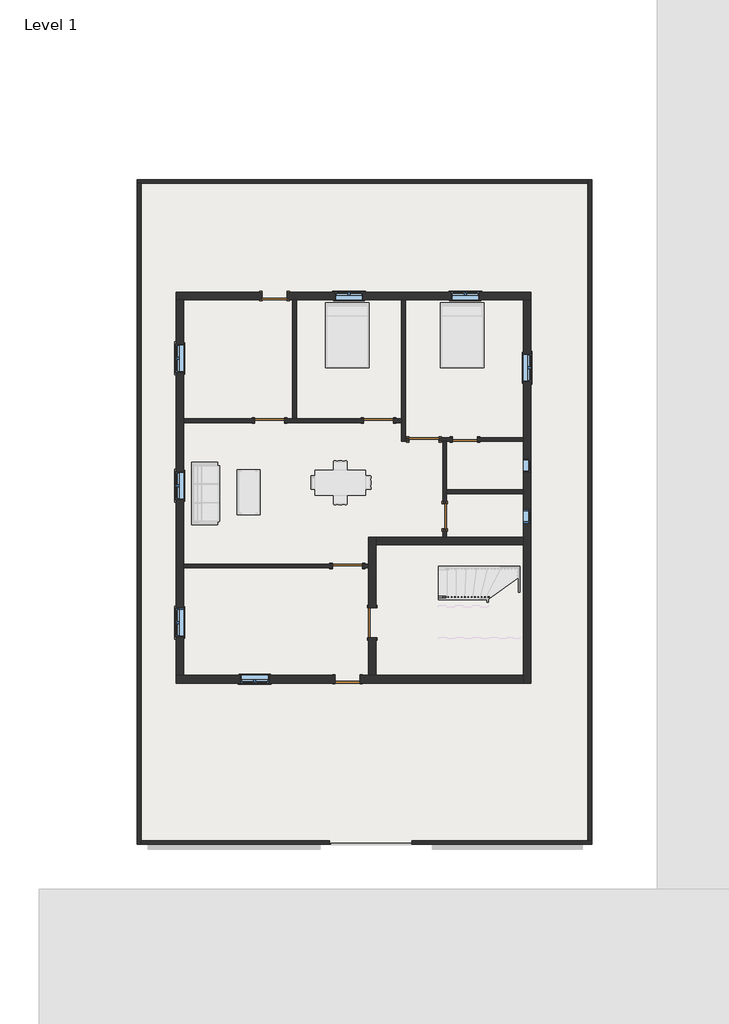
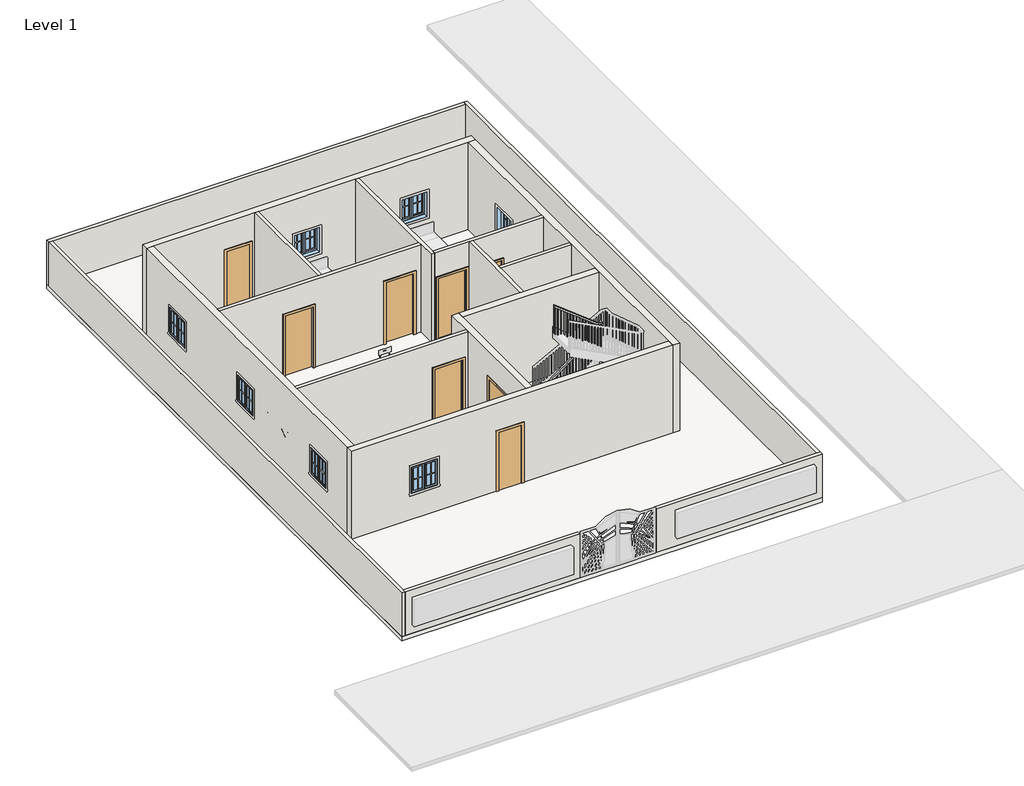
# One storey, part 1 of 2: 18 walls, 9 doors, 9 windows, 1 railing, 1 slab.
"""IFC4 building model written with IfcOpenShell, lengths in millimetres."""

from ifc_helpers import new_model, si_unit, frame, origin, origin_with_axes, place, context, project, spatial, polyline, outline, extrude, faceted_brep, transform, mapped, element, save
from components import door_85036156, door_d8f5dbb5, door_a1484949, door_e5f9f3c4, door_305aa2a5, door_0ca8825f, window_aa618e30, window_339605e1

model = new_model("IFC4")

# Units and contexts
model_context = context("Model", 3, world=origin())
ifc_project = project(units=[si_unit("LENGTHUNIT", "METRE", prefix="MILLI")], contexts=[model_context])

# Site, building, storey
site = spatial("IfcSite", under=ifc_project)
building = spatial("IfcBuilding", under=site)
storey = spatial("IfcBuildingStorey", under=building, Name="Level 1", Elevation=0.0)

# Doors
placement = place(None, origin())
door_shape = door_85036156(model_context)
element("IfcDoor", 1, ObjectType="Single-Flush : 30\" x 80\"", at=placement, inside=storey, context=model_context, shape_type="MappedRepresentation", body=[
    mapped(door_shape, transform((-3639.3817864, 7024.9034997, 0.0), x_axis=(1.0, 0.0, 0.0), y_axis=(0.0, 1.0, 0.0), z_axis=(0.0, 0.0, 1.0))),
])
door_2_shape = door_d8f5dbb5(model_context)
element("IfcDoor", 2, ObjectType="Single-Flush : 30\" x 80\"", at=placement, inside=storey, context=model_context, shape_type="MappedRepresentation", body=[
    mapped(door_2_shape, transform((2149.2782136, 2662.4534997, 0.0), x_axis=(-1.0, 0.0, 0.0), y_axis=(0.0, -1.0, 0.0), z_axis=(0.0, 0.0, 1.0))),
])
element("IfcDoor", 3, ObjectType="Single-Flush : 30\" x 80\"", at=placement, inside=storey, context=model_context, shape_type="MappedRepresentation", body=[
    mapped(door_2_shape, transform((1539.6782136, 322.4784997, 0.0), x_axis=(0.0, -1.0, 0.0), y_axis=(1.0, 0.0, 0.0), z_axis=(0.0, 0.0, 1.0))),
])
door_3_shape = door_a1484949(model_context)
element("IfcDoor", 4, ObjectType="Single-Flush : 30\" x 80\"", at=placement, inside=storey, context=model_context, shape_type="MappedRepresentation", body=[
    mapped(door_3_shape, transform((-1425.7717864, -4633.6965003, 0.0), x_axis=(-1.0, 0.0, 0.0), y_axis=(0.0, -1.0, 0.0), z_axis=(0.0, 0.0, 1.0))),
])
door_4_shape = door_e5f9f3c4(model_context)
element("IfcDoor", 5, ObjectType="Single-Flush : 36\" x 84\"", at=placement, inside=storey, context=model_context, shape_type="MappedRepresentation", body=[
    mapped(door_4_shape, transform((-477.0817864, 3233.9534997, 0.0), x_axis=(1.0, 0.0, 0.0), y_axis=(0.0, 1.0, 0.0), z_axis=(0.0, 0.0, 1.0))),
])
element("IfcDoor", 6, ObjectType="Single-Flush : 36\" x 84\"", at=placement, inside=storey, context=model_context, shape_type="MappedRepresentation", body=[
    mapped(door_4_shape, transform((-3791.7817864, 3233.9534997, 0.0), x_axis=(1.0, 0.0, 0.0), y_axis=(0.0, 1.0, 0.0), z_axis=(0.0, 0.0, 1.0))),
])
element("IfcDoor", 7, ObjectType="Single-Flush : 36\" x 84\"", at=placement, inside=storey, context=model_context, shape_type="MappedRepresentation", body=[
    mapped(door_4_shape, transform((-1425.7717864, -1188.1865003, 0.0), x_axis=(1.0, 0.0, 0.0), y_axis=(0.0, 1.0, 0.0), z_axis=(0.0, 0.0, 1.0))),
])
door_5_shape = door_305aa2a5(model_context)
element("IfcDoor", 8, ObjectType="Single-Flush : 36\" x 84\"", at=placement, inside=storey, context=model_context, shape_type="MappedRepresentation", body=[
    mapped(door_5_shape, transform((912.2982136, 2662.4534997, 0.0), x_axis=(-1.0, 0.0, 0.0), y_axis=(0.0, -1.0, 0.0), z_axis=(0.0, 0.0, 1.0))),
])
door_6_shape = door_0ca8825f(model_context)
element("IfcDoor", 9, ObjectType="Single-Flush : 36\" x 84\"", at=placement, inside=storey, context=model_context, shape_type="MappedRepresentation", body=[
    mapped(door_6_shape, transform((-663.7717864, -2910.9415003, 0.0), x_axis=(0.0, 1.0, 0.0), y_axis=(-1.0, 0.0, 0.0), z_axis=(0.0, 0.0, 1.0))),
])

# Railing
element("IfcRailing", 10, ObjectType="Handrail - Rectangular", at=placement, inside=storey, context=model_context, shape_type="SolidModel", body=[
    faceted_brep([(1342.8282136, -2108.9365003, 1083.7333333), (1342.8282136, -2108.9365003, 1019.4000346), (1342.8282136, -2159.7365003, 1019.4000346), (1342.8282136, -2159.7365003, 1083.7333333), (2794.3599055, -2108.9365003, 2211.6191036), (2845.1599055, -2108.9365003, 2186.7590024), (2845.1599055, -2159.7365003, 2186.7590024), (2794.3599055, -2159.7365003, 2211.6191036), (2794.3599055, -2108.9365003, 2414.6281882), (2845.1599055, -2108.9365003, 2363.8281882), (2845.1599055, -2159.7365003, 2363.8281882), (2794.3599055, -2159.7365003, 2414.6281882), (2921.3599055, -2108.9365003, 2414.6281882), (2921.3599055, -2108.9365003, 2363.8281882), (2870.5599055, -2159.7365003, 2363.8281882), (2870.5599055, -2159.7365003, 2414.6281882), (2921.3599055, -2235.9365003, 2414.6281882), (2921.3599055, -2265.0578342, 2363.8281882), (2870.5599055, -2265.0578342, 2363.8281882), (2870.5599055, -2235.9365003, 2414.6281882), (2921.3599055, -2362.9365003, 2631.5051451), (2921.3599055, -2413.7365003, 2617.7256424), (2870.5599055, -2413.7365003, 2617.7256424), (2870.5599055, -2362.9365003, 2631.5051451), (2921.3599055, -2362.9365003, 2834.5142297), (2921.3599055, -2413.7365003, 2783.7142297), (2870.5599055, -2413.7365003, 2783.7142297), (2870.5599055, -2362.9365003, 2834.5142297), (2921.3599055, -2489.9365003, 2834.5142297), (2921.3599055, -2489.9365003, 2783.7142297), (2870.5599055, -2439.1365003, 2783.7142297), (2870.5599055, -2439.1365003, 2834.5142297), (2794.3599055, -2489.9365003, 2834.5142297), (2776.9432376, -2489.9365003, 2783.7142297), (2776.9432376, -2439.1365003, 2783.7142297), (2794.3599055, -2439.1365003, 2834.5142297), (1342.8282136, -2489.9365003, 3962.4), (1342.8282136, -2439.1365003, 3962.4), (1342.8282136, -2439.1365003, 3898.0667013), (1342.8282136, -2489.9365003, 3898.0667013)], [[[0, 1, 2, 3]], [[1, 0, 4, 5]], [[2, 1, 5, 6]], [[3, 2, 6, 7]], [[0, 3, 7, 4]], [[5, 4, 8, 9]], [[6, 5, 9, 10]], [[7, 6, 10, 11]], [[4, 7, 11, 8]], [[9, 8, 12, 13]], [[10, 9, 13, 14]], [[11, 10, 14, 15]], [[8, 11, 15, 12]], [[13, 12, 16, 17]], [[14, 13, 17, 18]], [[15, 14, 18, 19]], [[12, 15, 19, 16]], [[17, 16, 20, 21]], [[18, 17, 21, 22]], [[19, 18, 22, 23]], [[16, 19, 23, 20]], [[21, 20, 24, 25]], [[22, 21, 25, 26]], [[23, 22, 26, 27]], [[20, 23, 27, 24]], [[25, 24, 28, 29]], [[26, 25, 29, 30]], [[27, 26, 30, 31]], [[24, 27, 31, 28]], [[29, 28, 32, 33]], [[30, 29, 33, 34]], [[31, 30, 34, 35]], [[28, 31, 35, 32]], [[36, 37, 38, 39]], [[33, 32, 36, 39]], [[34, 33, 39, 38]], [[35, 34, 38, 37]], [[32, 35, 37, 36]]]),
    extrude(outline(polyline([(3868.0292361, 1381.4849055), (3882.8316852, 1362.4349055), (2878.6666667, 1362.4349055), (2878.6666667, 1381.4849055), (3868.0292361, 1381.4849055)])), frame((0.0, -2474.0615003, 0.0), z_axis=(0.0, 1.0, 0.0), x_axis=(0.0, 0.0, 1.0)), (0.0, 0.0, 1.0), 19.05),
    extrude(outline(polyline([(3789.0828411, 1483.0849055), (3803.8852902, 1464.0349055), (2878.6666667, 1464.0349055), (2878.6666667, 1483.0849055), (3789.0828411, 1483.0849055)])), frame((0.0, -2474.0615003, 0.0), z_axis=(0.0, 1.0, 0.0), x_axis=(0.0, 0.0, 1.0)), (0.0, 0.0, 1.0), 19.05),
    extrude(outline(polyline([(3710.1364462, 1584.6849055), (3724.9388952, 1565.6349055), (2878.6666667, 1565.6349055), (2878.6666667, 1584.6849055), (3710.1364462, 1584.6849055)])), frame((0.0, -2474.0615003, 0.0), z_axis=(0.0, 1.0, 0.0), x_axis=(0.0, 0.0, 1.0)), (0.0, 0.0, 1.0), 19.05),
    extrude(outline(polyline([(3631.1900512, 1686.2849055), (3645.9925003, 1667.2349055), (2709.3333333, 1667.2349055), (2709.3333333, 1686.2849055), (3631.1900512, 1686.2849055)])), frame((0.0, -2474.0615003, 0.0), z_axis=(0.0, 1.0, 0.0), x_axis=(0.0, 0.0, 1.0)), (0.0, 0.0, 1.0), 19.05),
    extrude(outline(polyline([(3552.2436562, 1787.8849055), (3567.0461053, 1768.8349055), (2709.3333333, 1768.8349055), (2709.3333333, 1787.8849055), (3552.2436562, 1787.8849055)])), frame((0.0, -2474.0615003, 0.0), z_axis=(0.0, 1.0, 0.0), x_axis=(0.0, 0.0, 1.0)), (0.0, 0.0, 1.0), 19.05),
    extrude(outline(polyline([(3473.2972613, 1889.4849055), (3488.0997103, 1870.4349055), (2709.3333333, 1870.4349055), (2709.3333333, 1889.4849055), (3473.2972613, 1889.4849055)])), frame((0.0, -2474.0615003, 0.0), z_axis=(0.0, 1.0, 0.0), x_axis=(0.0, 0.0, 1.0)), (0.0, 0.0, 1.0), 19.05),
    extrude(outline(polyline([(3394.3508663, 1991.0849055), (3409.1533154, 1972.0349055), (2540.0, 1972.0349055), (2540.0, 1991.0849055), (3394.3508663, 1991.0849055)])), frame((0.0, -2474.0615003, 0.0), z_axis=(0.0, 1.0, 0.0), x_axis=(0.0, 0.0, 1.0)), (0.0, 0.0, 1.0), 19.05),
    extrude(outline(polyline([(3315.4044713, 2092.6849055), (3330.2069204, 2073.6349055), (2540.0, 2073.6349055), (2540.0, 2092.6849055), (3315.4044713, 2092.6849055)])), frame((0.0, -2474.0615003, 0.0), z_axis=(0.0, 1.0, 0.0), x_axis=(0.0, 0.0, 1.0)), (0.0, 0.0, 1.0), 19.05),
    extrude(outline(polyline([(3236.4580764, 2194.2849055), (3251.2605254, 2175.2349055), (2370.6666667, 2175.2349055), (2370.6666667, 2194.2849055), (3236.4580764, 2194.2849055)])), frame((0.0, -2474.0615003, 0.0), z_axis=(0.0, 1.0, 0.0), x_axis=(0.0, 0.0, 1.0)), (0.0, 0.0, 1.0), 19.05),
    extrude(outline(polyline([(3157.5116814, 2295.8849055), (3172.3141304, 2276.8349055), (2370.6666667, 2276.8349055), (2370.6666667, 2295.8849055), (3157.5116814, 2295.8849055)])), frame((0.0, -2474.0615003, 0.0), z_axis=(0.0, 1.0, 0.0), x_axis=(0.0, 0.0, 1.0)), (0.0, 0.0, 1.0), 19.05),
    extrude(outline(polyline([(3078.5652864, 2397.4849055), (3093.3677355, 2378.4349055), (2370.6666667, 2378.4349055), (2370.6666667, 2397.4849055), (3078.5652864, 2397.4849055)])), frame((0.0, -2474.0615003, 0.0), z_axis=(0.0, 1.0, 0.0), x_axis=(0.0, 0.0, 1.0)), (0.0, 0.0, 1.0), 19.05),
    extrude(outline(polyline([(2999.6188914, 2499.0849055), (3014.4213405, 2480.0349055), (2201.3333333, 2480.0349055), (2201.3333333, 2499.0849055), (2999.6188914, 2499.0849055)])), frame((0.0, -2474.0615003, 0.0), z_axis=(0.0, 1.0, 0.0), x_axis=(0.0, 0.0, 1.0)), (0.0, 0.0, 1.0), 19.05),
    extrude(outline(polyline([(2920.6724965, 2600.6849055), (2935.4749455, 2581.6349055), (2201.3333333, 2581.6349055), (2201.3333333, 2600.6849055), (2920.6724965, 2600.6849055)])), frame((0.0, -2474.0615003, 0.0), z_axis=(0.0, 1.0, 0.0), x_axis=(0.0, 0.0, 1.0)), (0.0, 0.0, 1.0), 19.05),
    extrude(outline(polyline([(2841.7261015, 2702.2849055), (2856.5285506, 2683.2349055), (2032.0, 2683.2349055), (2032.0, 2702.2849055), (2841.7261015, 2702.2849055)])), frame((0.0, -2474.0615003, 0.0), z_axis=(0.0, 1.0, 0.0), x_axis=(0.0, 0.0, 1.0)), (0.0, 0.0, 1.0), 19.05),
    extrude(outline(polyline([(2762.7797065, 2803.8849055), (2777.5821556, 2784.8349055), (2032.0, 2784.8349055), (2032.0, 2803.8849055), (2762.7797065, 2803.8849055)])), frame((0.0, -2474.0615003, 0.0), z_axis=(0.0, 1.0, 0.0), x_axis=(0.0, 0.0, 1.0)), (0.0, 0.0, 1.0), 19.05),
    extrude(outline(polyline([(2886.4349055, -2429.6115003), (2905.4849055, -2429.6115003), (2905.4849055, -2448.6615003), (2886.4349055, -2448.6615003), (2886.4349055, -2429.6115003)])), frame((0.0, 0.0, 1693.3333333), z_axis=(0.0, 0.0, 1.0), x_axis=(1.0, 0.0, 0.0)), (0.0, 0.0, 1.0), 1090.3808964),
    extrude(outline(polyline([(-2347.0615003, 2503.86524), (-2328.0115003, 2471.3336964), (-2328.0115003, 1524.0), (-2347.0615003, 1524.0), (-2347.0615003, 2503.86524)])), frame((2886.4349055, 0.0, 0.0), z_axis=(1.0, 0.0, 0.0), x_axis=(0.0, 1.0, 0.0)), (0.0, 0.0, 1.0), 19.05),
    extrude(outline(polyline([(-2245.4615003, 2330.3636744), (-2226.4115003, 2297.8321309), (-2226.4115003, 1354.6666667), (-2245.4615003, 1354.6666667), (-2245.4615003, 2330.3636744)])), frame((2886.4349055, 0.0, 0.0), z_axis=(1.0, 0.0, 0.0), x_axis=(0.0, 1.0, 0.0)), (0.0, 0.0, 1.0), 19.05),
    extrude(outline(polyline([(2857.3032136, -2143.8615003), (2857.3032136, -2124.8115003), (2876.3532136, -2124.8115003), (2876.3532136, -2143.8615003), (2857.3032136, -2143.8615003)])), frame((0.0, 0.0, 1185.3333333), z_axis=(0.0, 0.0, 1.0), x_axis=(1.0, 0.0, 0.0)), (0.0, 0.0, 1.0), 1178.4948549),
    extrude(outline(polyline([(2132.0507888, 2774.7532136), (2117.2483397, 2755.7032136), (1016.0, 2755.7032136), (1016.0, 2774.7532136), (2132.0507888, 2774.7532136)])), frame((0.0, -2143.8615003, 0.0), z_axis=(0.0, 1.0, 0.0), x_axis=(0.0, 0.0, 1.0)), (0.0, 0.0, 1.0), 19.05),
    extrude(outline(polyline([(2053.1043938, 2673.1532136), (2038.3019447, 2654.1032136), (1016.0, 2654.1032136), (1016.0, 2673.1532136), (2053.1043938, 2673.1532136)])), frame((0.0, -2143.8615003, 0.0), z_axis=(0.0, 1.0, 0.0), x_axis=(0.0, 0.0, 1.0)), (0.0, 0.0, 1.0), 19.05),
    extrude(outline(polyline([(1974.1579988, 2571.5532136), (1959.3555498, 2552.5032136), (846.6666667, 2552.5032136), (846.6666667, 2571.5532136), (1974.1579988, 2571.5532136)])), frame((0.0, -2143.8615003, 0.0), z_axis=(0.0, 1.0, 0.0), x_axis=(0.0, 0.0, 1.0)), (0.0, 0.0, 1.0), 19.05),
    extrude(outline(polyline([(1895.2116039, 2469.9532136), (1880.4091548, 2450.9032136), (846.6666667, 2450.9032136), (846.6666667, 2469.9532136), (1895.2116039, 2469.9532136)])), frame((0.0, -2143.8615003, 0.0), z_axis=(0.0, 1.0, 0.0), x_axis=(0.0, 0.0, 1.0)), (0.0, 0.0, 1.0), 19.05),
    extrude(outline(polyline([(1816.2652089, 2368.3532136), (1801.4627598, 2349.3032136), (677.3333333, 2349.3032136), (677.3333333, 2368.3532136), (1816.2652089, 2368.3532136)])), frame((0.0, -2143.8615003, 0.0), z_axis=(0.0, 1.0, 0.0), x_axis=(0.0, 0.0, 1.0)), (0.0, 0.0, 1.0), 19.05),
    extrude(outline(polyline([(1737.3188139, 2266.7532136), (1722.5163649, 2247.7032136), (677.3333333, 2247.7032136), (677.3333333, 2266.7532136), (1737.3188139, 2266.7532136)])), frame((0.0, -2143.8615003, 0.0), z_axis=(0.0, 1.0, 0.0), x_axis=(0.0, 0.0, 1.0)), (0.0, 0.0, 1.0), 19.05),
    extrude(outline(polyline([(1658.3724189, 2165.1532136), (1643.5699699, 2146.1032136), (508.0, 2146.1032136), (508.0, 2165.1532136), (1658.3724189, 2165.1532136)])), frame((0.0, -2143.8615003, 0.0), z_axis=(0.0, 1.0, 0.0), x_axis=(0.0, 0.0, 1.0)), (0.0, 0.0, 1.0), 19.05),
    extrude(outline(polyline([(1579.426024, 2063.5532136), (1564.6235749, 2044.5032136), (508.0, 2044.5032136), (508.0, 2063.5532136), (1579.426024, 2063.5532136)])), frame((0.0, -2143.8615003, 0.0), z_axis=(0.0, 1.0, 0.0), x_axis=(0.0, 0.0, 1.0)), (0.0, 0.0, 1.0), 19.05),
    extrude(outline(polyline([(1500.479629, 1961.9532136), (1485.6771799, 1942.9032136), (508.0, 1942.9032136), (508.0, 1961.9532136), (1500.479629, 1961.9532136)])), frame((0.0, -2143.8615003, 0.0), z_axis=(0.0, 1.0, 0.0), x_axis=(0.0, 0.0, 1.0)), (0.0, 0.0, 1.0), 19.05),
    extrude(outline(polyline([(1421.533234, 1860.3532136), (1406.730785, 1841.3032136), (338.6666667, 1841.3032136), (338.6666667, 1860.3532136), (1421.533234, 1860.3532136)])), frame((0.0, -2143.8615003, 0.0), z_axis=(0.0, 1.0, 0.0), x_axis=(0.0, 0.0, 1.0)), (0.0, 0.0, 1.0), 19.05),
    extrude(outline(polyline([(1342.5868391, 1758.7532136), (1327.78439, 1739.7032136), (338.6666667, 1739.7032136), (338.6666667, 1758.7532136), (1342.5868391, 1758.7532136)])), frame((0.0, -2143.8615003, 0.0), z_axis=(0.0, 1.0, 0.0), x_axis=(0.0, 0.0, 1.0)), (0.0, 0.0, 1.0), 19.05),
    extrude(outline(polyline([(1263.6404441, 1657.1532136), (1248.837995, 1638.1032136), (338.6666667, 1638.1032136), (338.6666667, 1657.1532136), (1263.6404441, 1657.1532136)])), frame((0.0, -2143.8615003, 0.0), z_axis=(0.0, 1.0, 0.0), x_axis=(0.0, 0.0, 1.0)), (0.0, 0.0, 1.0), 19.05),
    extrude(outline(polyline([(1184.6940491, 1555.5532136), (1169.8916001, 1536.5032136), (169.3333333, 1536.5032136), (169.3333333, 1555.5532136), (1184.6940491, 1555.5532136)])), frame((0.0, -2143.8615003, 0.0), z_axis=(0.0, 1.0, 0.0), x_axis=(0.0, 0.0, 1.0)), (0.0, 0.0, 1.0), 19.05),
    extrude(outline(polyline([(1105.7476541, 1453.9532136), (1090.9452051, 1434.9032136), (169.3333333, 1434.9032136), (169.3333333, 1453.9532136), (1105.7476541, 1453.9532136)])), frame((0.0, -2143.8615003, 0.0), z_axis=(0.0, 1.0, 0.0), x_axis=(0.0, 0.0, 1.0)), (0.0, 0.0, 1.0), 19.05),
    extrude(outline(polyline([(2886.4349055, -2455.0115003), (2905.4849055, -2455.0115003), (2905.4849055, -2474.0615003), (2886.4349055, -2474.0615003), (2886.4349055, -2455.0115003)])), frame((0.0, 0.0, 1862.6666667), z_axis=(0.0, 0.0, 1.0), x_axis=(1.0, 0.0, 0.0)), (0.0, 0.0, 1.0), 921.0475631),
    extrude(outline(polyline([(2886.4349055, -2143.8615003), (2886.4349055, -2124.8115003), (2905.4849055, -2124.8115003), (2905.4849055, -2143.8615003), (2886.4349055, -2143.8615003)])), frame((0.0, 0.0, 1185.3333333), z_axis=(0.0, 0.0, 1.0), x_axis=(1.0, 0.0, 0.0)), (0.0, 0.0, 1.0), 1178.4948549),
    extrude(outline(polyline([(3883.2642523, 1361.8782136), (3898.0667013, 1342.8282136), (2878.6666667, 1342.8282136), (2878.6666667, 1361.8782136), (3883.2642523, 1361.8782136)])), frame((0.0, -2474.0615003, 0.0), z_axis=(0.0, 1.0, 0.0), x_axis=(0.0, 0.0, 1.0)), (0.0, 0.0, 1.0), 19.05),
    extrude(outline(polyline([(1034.2024837, 1361.8782136), (1019.4000346, 1342.8282136), (169.3333333, 1342.8282136), (169.3333333, 1361.8782136), (1034.2024837, 1361.8782136)])), frame((0.0, -2143.8615003, 0.0), z_axis=(0.0, 1.0, 0.0), x_axis=(0.0, 0.0, 1.0)), (0.0, 0.0, 1.0), 19.05),
])

# Slab
element("IfcSlab", 11, ObjectType="Generic - 12\"", at=placement, inside=storey, context=model_context, shape_type="SweptSolid", body=[
    extrude(outline(polyline([(6012.9126462, 10570.8496734), (6012.9126462, -9660.2503266), (-7817.3873538, -9660.2503266), (-7817.3873538, 10570.8496734), (6012.9126462, 10570.8496734)])), frame((0.0, 0.0, -152.4), z_axis=(0.0, 0.0, 1.0), x_axis=(1.0, 0.0, 0.0)), (0.0, 0.0, 1.0), 152.4),
])

# Walls
element("IfcWall", 12, ObjectType="WALL4.5\"", at=placement, inside=storey, context=model_context, shape_type="Brep", body=[
    faceted_brep([(-3334.5817864, 3176.8034997, 2133.6), (-3334.5817864, 3176.8034997, 0.0), (-934.2817864, 3176.8034997, 0.0), (-934.2817864, 3176.8034997, 2133.6), (-19.8817864, 3176.8034997, 2133.6), (-19.8817864, 3176.8034997, 0.0), (227.7682136, 3176.8034997, 0.0), (227.7682136, 3176.8034997, 3048.0), (-6414.3317864, 3176.8034997, 3048.0), (-6414.3317864, 3176.8034997, 0.0), (-4248.9817864, 3176.8034997, 0.0), (-4248.9817864, 3176.8034997, 2133.6), (-934.2817864, 3291.1034997, 0.0), (-2972.6317864, 3291.1034997, 0.0), (-3086.9317864, 3291.1034997, 0.0), (-3334.5817864, 3291.1034997, 0.0), (-3334.5817864, 3291.1034997, 2133.6), (-4248.9817864, 3291.1034997, 2133.6), (-4248.9817864, 3291.1034997, 0.0), (-6414.3317864, 3291.1034997, 0.0), (-6414.3317864, 3291.1034997, 3048.0), (-3086.9317864, 3291.1034997, 3048.0), (-2972.6317864, 3291.1034997, 3048.0), (227.7682136, 3291.1034997, 3048.0), (227.7682136, 3291.1034997, 0.0), (-19.8817864, 3291.1034997, 0.0), (-19.8817864, 3291.1034997, 2133.6), (-934.2817864, 3291.1034997, 2133.6)], [[[0, 1, 2, 3, 4, 5, 6, 7, 8, 9, 10, 11]], [[12, 13, 14, 15, 16, 17, 18, 19, 20, 21, 22, 23, 24, 25, 26, 27]], [[6, 5, 25, 24]], [[10, 9, 19, 18]], [[2, 1, 15, 14, 13, 12]], [[9, 8, 20, 19]], [[7, 6, 24, 23]], [[26, 25, 5, 4]], [[27, 26, 4, 3]], [[12, 27, 3, 2]], [[16, 15, 1, 0]], [[17, 16, 0, 11]], [[18, 17, 11, 10]], [[8, 7, 23, 22, 21, 20]]]),
])
element("IfcWall", 13, ObjectType="WALL4.5\"", at=placement, inside=storey, context=model_context, shape_type="Brep", body=[
    faceted_brep([(227.7682136, 6910.6034997, 0.0), (227.7682136, 3291.1034997, 0.0), (227.7682136, 3176.8034997, 0.0), (227.7682136, 2605.3034997, 0.0), (227.7682136, 2605.3034997, 3048.0), (227.7682136, 3176.8034997, 3048.0), (227.7682136, 3291.1034997, 3048.0), (227.7682136, 6910.6034997, 3048.0), (342.0682136, 6910.6034997, 0.0), (342.0682136, 6910.6034997, 3048.0), (342.0682136, 2719.6034997, 3048.0), (342.0682136, 2605.3034997, 3048.0), (342.0682136, 2605.3034997, 0.0), (342.0682136, 2719.6034997, 0.0)], [[[0, 1, 2, 3, 4, 5, 6, 7]], [[8, 9, 10, 11, 12, 13]], [[3, 2, 1, 0, 8, 13, 12]], [[0, 7, 9, 8]], [[4, 3, 12, 11]], [[7, 6, 5, 4, 11, 10, 9]]]),
])
element("IfcWall", 14, ObjectType="WALL4.5\"", at=placement, inside=storey, context=model_context, shape_type="Brep", body=[
    faceted_brep([(1369.4982136, 2605.3034997, 0.0), (1482.5282136, 2605.3034997, 0.0), (1596.8282136, 2605.3034997, 0.0), (1768.2782136, 2605.3034997, 0.0), (1768.2782136, 2605.3034997, 2032.0), (2530.2782136, 2605.3034997, 2032.0), (2530.2782136, 2605.3034997, 0.0), (3933.6282136, 2605.3034997, 0.0), (3933.6282136, 2605.3034997, 3048.0), (1596.8282136, 2605.3034997, 3048.0), (1482.5282136, 2605.3034997, 3048.0), (342.0682136, 2605.3034997, 3048.0), (342.0682136, 2605.3034997, 0.0), (455.0982136, 2605.3034997, 0.0), (455.0982136, 2605.3034997, 2133.6), (1369.4982136, 2605.3034997, 2133.6), (1768.2782136, 2719.6034997, 2032.0), (1768.2782136, 2719.6034997, 0.0), (1369.4982136, 2719.6034997, 0.0), (1369.4982136, 2719.6034997, 2133.6), (455.0982136, 2719.6034997, 2133.6), (455.0982136, 2719.6034997, 0.0), (342.0682136, 2719.6034997, 0.0), (342.0682136, 2719.6034997, 3048.0), (3933.6282136, 2719.6034997, 3048.0), (3933.6282136, 2719.6034997, 0.0), (2530.2782136, 2719.6034997, 0.0), (2530.2782136, 2719.6034997, 2032.0)], [[[0, 1, 2, 3, 4, 5, 6, 7, 8, 9, 10, 11, 12, 13, 14, 15]], [[16, 17, 18, 19, 20, 21, 22, 23, 24, 25, 26, 27]], [[22, 21, 13, 12]], [[26, 25, 7, 6]], [[18, 17, 3, 2, 1, 0]], [[12, 11, 23, 22]], [[8, 7, 25, 24]], [[14, 13, 21, 20]], [[15, 14, 20, 19]], [[0, 15, 19, 18]], [[4, 3, 17, 16]], [[5, 4, 16, 27]], [[6, 5, 27, 26]], [[11, 10, 9, 8, 24, 23]]]),
])
element("IfcWall", 15, ObjectType="WALL4.5\"", at=placement, inside=storey, context=model_context, shape_type="SweptSolid", body=[
    extrude(outline(polyline([(-3086.9317864, 3291.1034997), (-3086.9317864, 6910.6034997), (-2972.6317864, 6910.6034997), (-2972.6317864, 3291.1034997), (-3086.9317864, 3291.1034997)])), origin_with_axes(), (0.0, 0.0, 1.0), 3048.0),
])
element("IfcWall", 16, ObjectType="WALL4.5\"", at=placement, inside=storey, context=model_context, shape_type="Brep", body=[
    faceted_brep([(1482.5282136, -58.5215003, 2032.0), (1482.5282136, -58.5215003, 0.0), (1482.5282136, -315.6965003, 0.0), (1482.5282136, -315.6965003, 3048.0), (1482.5282136, 2605.3034997, 3048.0), (1482.5282136, 2605.3034997, 0.0), (1482.5282136, 703.4784997, 0.0), (1482.5282136, 703.4784997, 2032.0), (1596.8282136, -315.6965003, 0.0), (1596.8282136, -58.5215003, 0.0), (1596.8282136, -58.5215003, 2032.0), (1596.8282136, 703.4784997, 2032.0), (1596.8282136, 703.4784997, 0.0), (1596.8282136, 1017.8034997, 0.0), (1596.8282136, 1132.1034997, 0.0), (1596.8282136, 2605.3034997, 0.0), (1596.8282136, 2605.3034997, 3048.0), (1596.8282136, 1132.1034997, 3048.0), (1596.8282136, 1017.8034997, 3048.0), (1596.8282136, -315.6965003, 3048.0)], [[[0, 1, 2, 3, 4, 5, 6, 7]], [[8, 9, 10, 11, 12, 13, 14, 15, 16, 17, 18, 19]], [[6, 5, 15, 14, 13, 12]], [[2, 1, 9, 8]], [[5, 4, 16, 15]], [[3, 2, 8, 19]], [[10, 9, 1, 0]], [[11, 10, 0, 7]], [[12, 11, 7, 6]], [[4, 3, 19, 18, 17, 16]]]),
])
element("IfcWall", 17, ObjectType="WALL4.5\"", at=placement, inside=storey, context=model_context, shape_type="SweptSolid", body=[
    extrude(outline(polyline([(3933.6282136, 1017.8034997), (1596.8282136, 1017.8034997), (1596.8282136, 1132.1034997), (3933.6282136, 1132.1034997), (3933.6282136, 1017.8034997)])), origin_with_axes(), (0.0, 0.0, 1.0), 3048.0),
])
element("IfcWall", 18, ObjectType="WALL4.5\"", at=placement, inside=storey, context=model_context, shape_type="SweptSolid", body=[
    extrude(outline(polyline([(2133.6, -968.5717864), (0.0, -968.5717864), (0.0, -778.0717864), (3048.0, -778.0717864), (3048.0, -6414.3317864), (0.0, -6414.3317864), (0.0, -1882.9717864), (2133.6, -1882.9717864), (2133.6, -968.5717864)])), frame((0.0, -1245.3365003, 0.0), z_axis=(0.0, 1.0, 0.0), x_axis=(0.0, 0.0, 1.0)), (0.0, 0.0, 1.0), 114.3),
])
element("IfcWall", 19, ObjectType="WALL4.5\"", at=placement, inside=storey, context=model_context, shape_type="Brep", body=[
    faceted_brep([(-7817.3873538, 10456.5496734, 0.0), (-7703.0873538, 10456.5496734, 0.0), (5898.6126462, 10456.5496734, 0.0), (5898.6126462, 10456.5496734, 1524.0), (-7703.0873538, 10456.5496734, 1524.0), (-7817.3873538, 10456.5496734, 1524.0), (-7817.3873538, 10570.8496734, 0.0), (-7817.3873538, 10570.8496734, 1524.0), (5898.6126462, 10570.8496734, 1524.0), (5898.6126462, 10570.8496734, 0.0)], [[[0, 1, 2, 3, 4, 5]], [[6, 7, 8, 9]], [[2, 1, 0, 6, 9]], [[5, 4, 3, 8, 7]], [[0, 5, 7, 6]], [[3, 2, 9, 8]]]),
])
element("IfcWall", 20, ObjectType="WALL4.5\"", at=placement, inside=storey, context=model_context, shape_type="Brep", body=[
    faceted_brep([(-7703.0873538, -9660.2503266, 0.0), (-7703.0873538, -9545.9503266, 0.0), (-7703.0873538, 10456.5496734, 0.0), (-7703.0873538, 10456.5496734, 1524.0), (-7703.0873538, -9545.9503266, 1524.0), (-7703.0873538, -9660.2503266, 1524.0), (-7817.3873538, -9660.2503266, 0.0), (-7817.3873538, -9660.2503266, 1524.0), (-7817.3873538, 10456.5496734, 1524.0), (-7817.3873538, 10456.5496734, 0.0)], [[[0, 1, 2, 3, 4, 5]], [[6, 7, 8, 9]], [[2, 1, 0, 6, 9]], [[5, 4, 3, 8, 7]], [[0, 5, 7, 6]], [[3, 2, 9, 8]]]),
])
element("IfcWall", 21, ObjectType="WALL4.5\"", at=placement, inside=storey, context=model_context, shape_type="Brep", body=[
    faceted_brep([(6012.9126462, -9545.9503266, 0.0), (5898.6126462, -9545.9503266, 0.0), (545.5626462, -9545.9503266, 0.0), (545.5626462, -9545.9503266, 1524.0), (5898.6126462, -9545.9503266, 1524.0), (6012.9126462, -9545.9503266, 1524.0), (6012.9126462, -9660.2503266, 0.0), (6012.9126462, -9660.2503266, 1524.0), (545.5626462, -9660.2503266, 1524.0), (545.5626462, -9660.2503266, 0.0)], [[[0, 1, 2, 3, 4, 5]], [[6, 7, 8, 9]], [[2, 1, 0, 6, 9]], [[3, 2, 9, 8]], [[5, 4, 3, 8, 7]], [[0, 5, 7, 6]]]),
])
element("IfcWall", 22, ObjectType="WALL4.5\"", at=placement, inside=storey, context=model_context, shape_type="Brep", body=[
    faceted_brep([(5898.6126462, 10570.8496734, 0.0), (5898.6126462, 10456.5496734, 0.0), (5898.6126462, -9545.9503266, 0.0), (5898.6126462, -9545.9503266, 1524.0), (5898.6126462, 10456.5496734, 1524.0), (5898.6126462, 10570.8496734, 1524.0), (6012.9126462, 10570.8496734, 0.0), (6012.9126462, 10570.8496734, 1524.0), (6012.9126462, -9545.9503266, 1524.0), (6012.9126462, -9545.9503266, 0.0)], [[[0, 1, 2, 3, 4, 5]], [[6, 7, 8, 9]], [[2, 1, 0, 6, 9]], [[5, 4, 3, 8, 7]], [[0, 5, 7, 6]], [[3, 2, 9, 8]]]),
])
element("IfcWall", 23, ObjectType="WALL4.5\"", at=placement, inside=storey, context=model_context, shape_type="SweptSolid", body=[
    extrude(outline(polyline([(-7703.0873538, -9545.9503266), (-1969.0373538, -9545.9503266), (-1969.0373538, -9660.2503266), (-7703.0873538, -9660.2503266), (-7703.0873538, -9545.9503266)])), origin_with_axes(), (0.0, 0.0, 1.0), 1524.0),
])
element("IfcWall", 24, ObjectType="WALL9\"", at=placement, inside=storey, context=model_context, shape_type="Brep", body=[
    faceted_brep([(-3258.3817864, 6910.6034997, 2032.0), (-3258.3817864, 6910.6034997, 0.0), (-3086.9317864, 6910.6034997, 0.0), (-2972.6317864, 6910.6034997, 0.0), (227.7682136, 6910.6034997, 0.0), (342.0682136, 6910.6034997, 0.0), (3933.6282136, 6910.6034997, 0.0), (4162.2282136, 6910.6034997, 0.0), (4162.2282136, 6910.6034997, 3048.0), (3933.6282136, 6910.6034997, 3048.0), (342.0682136, 6910.6034997, 3048.0), (227.7682136, 6910.6034997, 3048.0), (-2972.6317864, 6910.6034997, 3048.0), (-3086.9317864, 6910.6034997, 3048.0), (-6414.3317864, 6910.6034997, 3048.0), (-6642.9317864, 6910.6034997, 3048.0), (-6642.9317864, 6910.6034997, 0.0), (-6414.3317864, 6910.6034997, 0.0), (-4020.3817864, 6910.6034997, 0.0), (-4020.3817864, 6910.6034997, 2032.0), (-940.6317864, 6910.6034997, 1828.8), (-940.6317864, 6910.6034997, 914.4), (-1804.2317864, 6910.6034997, 914.4), (-1804.2317864, 6910.6034997, 1828.8), (2598.2232136, 6910.6034997, 1828.8), (2598.2232136, 6910.6034997, 914.4), (1734.6232136, 6910.6034997, 914.4), (1734.6232136, 6910.6034997, 1828.8), (4162.2282136, 7139.2034997, 0.0), (-3258.3817864, 7139.2034997, 0.0), (-3258.3817864, 7139.2034997, 2032.0), (-4020.3817864, 7139.2034997, 2032.0), (-4020.3817864, 7139.2034997, 0.0), (-6642.9317864, 7139.2034997, 0.0), (-6642.9317864, 7139.2034997, 3048.0), (4162.2282136, 7139.2034997, 3048.0), (-940.6317864, 7139.2034997, 1828.8), (-1804.2317864, 7139.2034997, 1828.8), (-1804.2317864, 7139.2034997, 914.4), (-940.6317864, 7139.2034997, 914.4), (2598.2232136, 7139.2034997, 1828.8), (1734.6232136, 7139.2034997, 1828.8), (1734.6232136, 7139.2034997, 914.4), (2598.2232136, 7139.2034997, 914.4)], [[[0, 1, 2, 3, 4, 5, 6, 7, 8, 9, 10, 11, 12, 13, 14, 15, 16, 17, 18, 19], [20, 21, 22, 23], [24, 25, 26, 27]], [[28, 29, 30, 31, 32, 33, 34, 35], [36, 37, 38, 39], [40, 41, 42, 43]], [[18, 17, 16, 33, 32]], [[7, 6, 5, 4, 3, 2, 1, 29, 28]], [[8, 7, 28, 35]], [[16, 15, 34, 33]], [[30, 29, 1, 0]], [[31, 30, 0, 19]], [[32, 31, 19, 18]], [[21, 20, 36, 39]], [[22, 21, 39, 38]], [[23, 22, 38, 37]], [[20, 23, 37, 36]], [[25, 24, 40, 43]], [[26, 25, 43, 42]], [[27, 26, 42, 41]], [[24, 27, 41, 40]], [[15, 14, 13, 12, 11, 10, 9, 8, 35, 34]]]),
])
element("IfcWall", 25, ObjectType="WALL9\"", at=placement, inside=storey, context=model_context, shape_type="Brep", body=[
    faceted_brep([(3933.6282136, 6910.6034997, 0.0), (3933.6282136, 2719.6034997, 0.0), (3933.6282136, 2605.3034997, 0.0), (3933.6282136, 1132.1034997, 0.0), (3933.6282136, 1017.8034997, 0.0), (3933.6282136, -315.6965003, 0.0), (3933.6282136, -544.2965003, 0.0), (3933.6282136, -4519.3965003, 0.0), (3933.6282136, -4747.9965003, 0.0), (3933.6282136, -4747.9965003, 3048.0), (3933.6282136, -4519.3965003, 3048.0), (3933.6282136, -544.2965003, 3048.0), (3933.6282136, -315.6965003, 3048.0), (3933.6282136, 1017.8034997, 3048.0), (3933.6282136, 1132.1034997, 3048.0), (3933.6282136, 2605.3034997, 3048.0), (3933.6282136, 2719.6034997, 3048.0), (3933.6282136, 6910.6034997, 3048.0), (3933.6282136, 1665.5034997, 1524.0), (3933.6282136, 1665.5034997, 914.4), (3933.6282136, 2071.9034997, 914.4), (3933.6282136, 2071.9034997, 1524.0), (3933.6282136, 119.2784997, 1524.0), (3933.6282136, 119.2784997, 914.4), (3933.6282136, 525.6784997, 914.4), (3933.6282136, 525.6784997, 1524.0), (3933.6282136, 4411.8784997, 1828.8), (3933.6282136, 4411.8784997, 914.4), (3933.6282136, 5275.4784997, 914.4), (3933.6282136, 5275.4784997, 1828.8), (4162.2282136, 6910.6034997, 0.0), (4162.2282136, 6910.6034997, 3048.0), (4162.2282136, -4747.9965003, 3048.0), (4162.2282136, -4747.9965003, 0.0), (4162.2282136, 1665.5034997, 1524.0), (4162.2282136, 2071.9034997, 1524.0), (4162.2282136, 2071.9034997, 914.4), (4162.2282136, 1665.5034997, 914.4), (4162.2282136, 119.2784997, 1524.0), (4162.2282136, 525.6784997, 1524.0), (4162.2282136, 525.6784997, 914.4), (4162.2282136, 119.2784997, 914.4), (4162.2282136, 4411.8784997, 1828.8), (4162.2282136, 5275.4784997, 1828.8), (4162.2282136, 5275.4784997, 914.4), (4162.2282136, 4411.8784997, 914.4)], [[[0, 1, 2, 3, 4, 5, 6, 7, 8, 9, 10, 11, 12, 13, 14, 15, 16, 17], [18, 19, 20, 21], [22, 23, 24, 25], [26, 27, 28, 29]], [[30, 31, 32, 33], [34, 35, 36, 37], [38, 39, 40, 41], [42, 43, 44, 45]], [[8, 7, 6, 5, 4, 3, 2, 1, 0, 30, 33]], [[0, 17, 31, 30]], [[9, 8, 33, 32]], [[19, 18, 34, 37]], [[20, 19, 37, 36]], [[21, 20, 36, 35]], [[18, 21, 35, 34]], [[23, 22, 38, 41]], [[24, 23, 41, 40]], [[25, 24, 40, 39]], [[22, 25, 39, 38]], [[27, 26, 42, 45]], [[28, 27, 45, 44]], [[29, 28, 44, 43]], [[26, 29, 43, 42]], [[17, 16, 15, 14, 13, 12, 11, 10, 9, 32, 31]]]),
])
element("IfcWall", 26, ObjectType="WALL9\"", at=placement, inside=storey, context=model_context, shape_type="Brep", body=[
    faceted_brep([(-1806.7717864, -4519.3965003, 2032.0), (-1806.7717864, -4519.3965003, 0.0), (-6414.3317864, -4519.3965003, 0.0), (-6642.9317864, -4519.3965003, 0.0), (-6642.9317864, -4519.3965003, 3048.0), (-6414.3317864, -4519.3965003, 3048.0), (-778.0717864, -4519.3965003, 3048.0), (-549.4717864, -4519.3965003, 3048.0), (3933.6282136, -4519.3965003, 3048.0), (3933.6282136, -4519.3965003, 0.0), (-549.4717864, -4519.3965003, 0.0), (-778.0717864, -4519.3965003, 0.0), (-1044.7717864, -4519.3965003, 0.0), (-1044.7717864, -4519.3965003, 2032.0), (-4674.4317864, -4519.3965003, 1828.8), (-4674.4317864, -4519.3965003, 914.4), (-3810.8317864, -4519.3965003, 914.4), (-3810.8317864, -4519.3965003, 1828.8), (-6642.9317864, -4747.9965003, 0.0), (-1806.7717864, -4747.9965003, 0.0), (-1806.7717864, -4747.9965003, 2032.0), (-1044.7717864, -4747.9965003, 2032.0), (-1044.7717864, -4747.9965003, 0.0), (3933.6282136, -4747.9965003, 0.0), (3933.6282136, -4747.9965003, 3048.0), (-6642.9317864, -4747.9965003, 3048.0), (-4674.4317864, -4747.9965003, 1828.8), (-3810.8317864, -4747.9965003, 1828.8), (-3810.8317864, -4747.9965003, 914.4), (-4674.4317864, -4747.9965003, 914.4)], [[[0, 1, 2, 3, 4, 5, 6, 7, 8, 9, 10, 11, 12, 13], [14, 15, 16, 17]], [[18, 19, 20, 21, 22, 23, 24, 25], [26, 27, 28, 29]], [[3, 2, 1, 19, 18]], [[12, 11, 10, 9, 23, 22]], [[9, 8, 24, 23]], [[4, 3, 18, 25]], [[15, 14, 26, 29]], [[16, 15, 29, 28]], [[17, 16, 28, 27]], [[14, 17, 27, 26]], [[8, 7, 6, 5, 4, 25, 24]], [[20, 19, 1, 0]], [[21, 20, 0, 13]], [[22, 21, 13, 12]]]),
])
element("IfcWall", 27, ObjectType="WALL9\"", at=placement, inside=storey, context=model_context, shape_type="Brep", body=[
    faceted_brep([(-6414.3317864, -4519.3965003, 0.0), (-6414.3317864, -1245.3365003, 0.0), (-6414.3317864, -1131.0365003, 0.0), (-6414.3317864, 3176.8034997, 0.0), (-6414.3317864, 3291.1034997, 0.0), (-6414.3317864, 6910.6034997, 0.0), (-6414.3317864, 6910.6034997, 3048.0), (-6414.3317864, 3291.1034997, 3048.0), (-6414.3317864, 3176.8034997, 3048.0), (-6414.3317864, -1131.0365003, 3048.0), (-6414.3317864, -1245.3365003, 3048.0), (-6414.3317864, -4519.3965003, 3048.0), (-6414.3317864, 5561.2284997, 1828.8), (-6414.3317864, 5561.2284997, 914.4), (-6414.3317864, 4697.6284997, 914.4), (-6414.3317864, 4697.6284997, 1828.8), (-6414.3317864, 1684.5534997, 1828.8), (-6414.3317864, 1684.5534997, 914.4), (-6414.3317864, 820.9534997, 914.4), (-6414.3317864, 820.9534997, 1828.8), (-6414.3317864, -2479.1415003, 1828.8), (-6414.3317864, -2479.1415003, 914.4), (-6414.3317864, -3342.7415003, 914.4), (-6414.3317864, -3342.7415003, 1828.8), (-6642.9317864, -4519.3965003, 0.0), (-6642.9317864, -4519.3965003, 3048.0), (-6642.9317864, 6910.6034997, 3048.0), (-6642.9317864, 6910.6034997, 0.0), (-6642.9317864, 5561.2284997, 1828.8), (-6642.9317864, 4697.6284997, 1828.8), (-6642.9317864, 4697.6284997, 914.4), (-6642.9317864, 5561.2284997, 914.4), (-6642.9317864, 1684.5534997, 1828.8), (-6642.9317864, 820.9534997, 1828.8), (-6642.9317864, 820.9534997, 914.4), (-6642.9317864, 1684.5534997, 914.4), (-6642.9317864, -2479.1415003, 1828.8), (-6642.9317864, -3342.7415003, 1828.8), (-6642.9317864, -3342.7415003, 914.4), (-6642.9317864, -2479.1415003, 914.4)], [[[0, 1, 2, 3, 4, 5, 6, 7, 8, 9, 10, 11], [12, 13, 14, 15], [16, 17, 18, 19], [20, 21, 22, 23]], [[24, 25, 26, 27], [28, 29, 30, 31], [32, 33, 34, 35], [36, 37, 38, 39]], [[5, 4, 3, 2, 1, 0, 24, 27]], [[0, 11, 25, 24]], [[6, 5, 27, 26]], [[13, 12, 28, 31]], [[14, 13, 31, 30]], [[15, 14, 30, 29]], [[12, 15, 29, 28]], [[17, 16, 32, 35]], [[18, 17, 35, 34]], [[19, 18, 34, 33]], [[16, 19, 33, 32]], [[21, 20, 36, 39]], [[22, 21, 39, 38]], [[23, 22, 38, 37]], [[20, 23, 37, 36]], [[11, 10, 9, 8, 7, 6, 26, 25]]]),
])
element("IfcWall", 28, ObjectType="WALL9\"", at=placement, inside=storey, context=model_context, shape_type="Brep", body=[
    faceted_brep([(-549.4717864, -2453.7415003, 2133.6), (-549.4717864, -2453.7415003, 0.0), (-549.4717864, -544.2965003, 0.0), (-549.4717864, -315.6965003, 0.0), (-549.4717864, -315.6965003, 3048.0), (-549.4717864, -544.2965003, 3048.0), (-549.4717864, -4519.3965003, 3048.0), (-549.4717864, -4519.3965003, 0.0), (-549.4717864, -3368.1415003, 0.0), (-549.4717864, -3368.1415003, 2133.6), (-778.0717864, -315.6965003, 0.0), (-778.0717864, -1131.0365003, 0.0), (-778.0717864, -1245.3365003, 0.0), (-778.0717864, -2453.7415003, 0.0), (-778.0717864, -2453.7415003, 2133.6), (-778.0717864, -3368.1415003, 2133.6), (-778.0717864, -3368.1415003, 0.0), (-778.0717864, -4519.3965003, 0.0), (-778.0717864, -4519.3965003, 3048.0), (-778.0717864, -1245.3365003, 3048.0), (-778.0717864, -1131.0365003, 3048.0), (-778.0717864, -315.6965003, 3048.0)], [[[0, 1, 2, 3, 4, 5, 6, 7, 8, 9]], [[10, 11, 12, 13, 14, 15, 16, 17, 18, 19, 20, 21]], [[8, 7, 17, 16]], [[3, 2, 1, 13, 12, 11, 10]], [[7, 6, 18, 17]], [[4, 3, 10, 21]], [[14, 13, 1, 0]], [[15, 14, 0, 9]], [[16, 15, 9, 8]], [[6, 5, 4, 21, 20, 19, 18]]]),
])
element("IfcWall", 29, ObjectType="WALL9\"", at=placement, inside=storey, context=model_context, shape_type="Brep", body=[
    faceted_brep([(-549.4717864, -544.2965003, 0.0), (3933.6282136, -544.2965003, 0.0), (3933.6282136, -544.2965003, 3048.0), (-549.4717864, -544.2965003, 3048.0), (-549.4717864, -315.6965003, 0.0), (-549.4717864, -315.6965003, 3048.0), (1482.5282136, -315.6965003, 3048.0), (1596.8282136, -315.6965003, 3048.0), (3933.6282136, -315.6965003, 3048.0), (3933.6282136, -315.6965003, 0.0), (1596.8282136, -315.6965003, 0.0), (1482.5282136, -315.6965003, 0.0)], [[[0, 1, 2, 3]], [[4, 5, 6, 7, 8, 9, 10, 11]], [[1, 0, 4, 11, 10, 9]], [[0, 3, 5, 4]], [[2, 1, 9, 8]], [[3, 2, 8, 7, 6, 5]]]),
])

# Windows
window_shape = window_aa618e30(model_context)
element("IfcWindow", 30, ObjectType="Fixed : 16\" x 24\"", at=placement, inside=storey, context=model_context, shape_type="MappedRepresentation", body=[
    mapped(window_shape, transform((4047.9282136, 1830.6034997, 0.0), x_axis=(0.0, -1.0, 0.0), y_axis=(1.0, 0.0, 0.0), z_axis=(0.0, 0.0, 1.0))),
])
element("IfcWindow", 31, ObjectType="Fixed : 16\" x 24\"", at=placement, inside=storey, context=model_context, shape_type="MappedRepresentation", body=[
    mapped(window_shape, transform((4047.9282136, 284.3784997, 0.0), x_axis=(0.0, -1.0, 0.0), y_axis=(1.0, 0.0, 0.0), z_axis=(0.0, 0.0, 1.0))),
])
window_2_shape = window_339605e1(model_context)
element("IfcWindow", 32, ObjectType="Window-Casement-Double : 34\" x 36\"", at=placement, inside=storey, context=model_context, shape_type="MappedRepresentation", body=[
    mapped(window_2_shape, transform((-1372.4317864, 7024.9034997, 0.0), x_axis=(1.0, 0.0, 0.0), y_axis=(0.0, 1.0, 0.0), z_axis=(0.0, 0.0, 1.0))),
])
element("IfcWindow", 33, ObjectType="Window-Casement-Double : 34\" x 36\"", at=placement, inside=storey, context=model_context, shape_type="MappedRepresentation", body=[
    mapped(window_2_shape, transform((2166.4232136, 7024.9034997, 0.0), x_axis=(1.0, 0.0, 0.0), y_axis=(0.0, 1.0, 0.0), z_axis=(0.0, 0.0, 1.0))),
])
element("IfcWindow", 34, ObjectType="Window-Casement-Double : 34\" x 36\"", at=placement, inside=storey, context=model_context, shape_type="MappedRepresentation", body=[
    mapped(window_2_shape, transform((-6528.6317864, 5129.4284997, 0.0), x_axis=(0.0, 1.0, 0.0), y_axis=(-1.0, 0.0, 0.0), z_axis=(0.0, 0.0, 1.0))),
])
element("IfcWindow", 35, ObjectType="Window-Casement-Double : 34\" x 36\"", at=placement, inside=storey, context=model_context, shape_type="MappedRepresentation", body=[
    mapped(window_2_shape, transform((-6528.6317864, 1252.7534997, 0.0), x_axis=(0.0, 1.0, 0.0), y_axis=(-1.0, 0.0, 0.0), z_axis=(0.0, 0.0, 1.0))),
])
element("IfcWindow", 36, ObjectType="Window-Casement-Double : 34\" x 36\"", at=placement, inside=storey, context=model_context, shape_type="MappedRepresentation", body=[
    mapped(window_2_shape, transform((4047.9282136, 4843.6784997, 0.0), x_axis=(0.0, -1.0, 0.0), y_axis=(1.0, 0.0, 0.0), z_axis=(0.0, 0.0, 1.0))),
])
element("IfcWindow", 37, ObjectType="Window-Casement-Double : 34\" x 36\"", at=placement, inside=storey, context=model_context, shape_type="MappedRepresentation", body=[
    mapped(window_2_shape, transform((-6528.6317864, -2910.9415003, 0.0), x_axis=(0.0, 1.0, 0.0), y_axis=(-1.0, 0.0, 0.0), z_axis=(0.0, 0.0, 1.0))),
])
element("IfcWindow", 38, ObjectType="Window-Casement-Double : 34\" x 36\"", at=placement, inside=storey, context=model_context, shape_type="MappedRepresentation", body=[
    mapped(window_2_shape, transform((-4242.6317864, -4633.6965003, 0.0), x_axis=(-1.0, 0.0, 0.0), y_axis=(0.0, -1.0, 0.0), z_axis=(0.0, 0.0, 1.0))),
])

save(model, "model.ifc")

# Revit data of these elements
# Type "Single-Flush : 30\" x 80\""
#   Type Mark = "5"
#   Construction Type Id = "MDOOR"
#   Assembly Code = "C1020"
#   Analytic Construction = "Metal"
#   Thickness = 0' - 2"
#   Heat Transfer Coefficient (U) = 0.651978 BTU/(h·ft²·°F)
#   Height = 6' - 8"
#   Trim Projection Ext = 0' - 1"
#   Trim Projection Int = 0' - 1"
#   Trim Width = 0' - 3"
#   Width = 2' - 6"
#   Define Thermal Properties by = 1
#   Define Thermal Properties by = 1
#   Door Material = Door - Panel
#   Frame Material = Door - Frame
#   Visual Light Transmittance = 0
#   Solar Heat Gain Coefficient = 0
#   Function = (empty or 0)
#   Wall Closure = (empty or 0)
# Type "Single-Flush : 36\" x 84\""
#   Type Mark = "1"
#   Construction Type Id = "MDOOR"
#   Assembly Code = "C1020"
#   Analytic Construction = "Metal"
#   Thickness = 0' - 2"
#   Heat Transfer Coefficient (U) = 0.651978 BTU/(h·ft²·°F)
#   Height = 7' - 0"
#   Trim Projection Ext = 0' - 1"
#   Trim Projection Int = 0' - 1"
#   Trim Width = 0' - 3"
#   Width = 3' - 0"
#   Define Thermal Properties by = 1
#   Define Thermal Properties by = 1
#   Door Material = Door - Panel
#   Frame Material = Door - Frame
#   Visual Light Transmittance = 0
#   Solar Heat Gain Coefficient = 0
#   Function = (empty or 0)
#   Wall Closure = (empty or 0)
# Type "Handrail - Rectangular"
#   Assembly Code = "C2010400"
#   built-in parameter 1008612 = 0.0416667 (stored number, unit not read)
#   built-in parameter 1008611 = 0.0416667 (stored number, unit not read)
#   built-in parameter 1008609 = 0.333333 (stored number, unit not read)
#   built-in parameter 1008604 = 0.166667 (stored number, unit not read)
#   built-in parameter 1008603 = 0.166667 (stored number, unit not read)
#   Railing Height = 3' - 0"
#   built-in parameter 1008630 = 2
#   built-in parameter 1008610 = 2
#   built-in parameter 1008618 = Baluster - Square : 3/4"
# Type "Generic - 12\""
#   Assembly Code = "B1010"
#   Function = 0
#   Layers, outside or top first: 0' - 6" no material (function 1)
# Type "WALL4.5\""
#   Assembly Code = "B2010"
#   Layers, outside or top first: 0' - 4 1/2" no material (function 1)
# Type "WALL9\""
#   Assembly Code = "B2010"
#   Layers, outside or top first: 0' - 9" no material (function 1)
# Type "Fixed : 16\" x 24\""
#   Type Mark = "4"
#   Construction Type Id = "GSP4R"
#   Assembly Code = "B2020100"
#   Analytic Construction = "1/8 in Pilkington single glazing"
#   Visual Light Transmittance = 0.9
#   Solar Heat Gain Coefficient = 0.78
#   Heat Transfer Coefficient (U) = 0.6496 BTU/(h·ft²·°F)
#   Height = 2' - 0"
#   Default Sill Height = 3' - 0"
#   Width = 1' - 4"
#   Window Inset = 0' - 0 3/4"
#   Define Thermal Properties by = 1
#   Define Thermal Properties by = 1
#   Glass Pane Material = Glass
#   Sash Material = Sash
#   Wall Closure = (empty or 0)
# Type "Window-Casement-Double : 34\" x 36\""
#   Type Mark = "14"
#   Fire Rating = "0.5h"
#   Assembly Code = "B2020100"
#   Analytic Construction = "Double glazing - domestic"
#   Frame Extension [instance default] = 0' - 0 1/4"
#   Window Inset [instance default] = 0' - 0"
#   Wall Thickness [instance default] = 0' - 6"
#   Interior Wall Closure [instance default] = 0' - 2 1/4"
#   Half Width = 1' - 5"
#   Visual Light Transmittance = 0.81
#   Thermal Resistance (R) = 1.8146 (h·ft²·°F)/BTU
#   Solar Heat Gain Coefficient = 0.76
#   Rough Width = 2' - 10 1/2"
#   Rough Height = 3' - 0 1/2"
#   Height = 3' - 0"
#   Heat Transfer Coefficient (U) = 0.5511 BTU/(h·ft²·°F)
#   Exterior Wall Closure [instance default] = 0' - 1 1/4"
#   Extension Jamb [instance default] = 0' - 2 1/4"
#   Default Sill Height = 3' - 0"
#   Width = 2' - 10"
#   Define Thermal Properties by = 0
#   Muntin Visibility = yes
#   Interior Trim Visibility [instance default] = yes
#   Exterior Trim Visibility [instance default] = yes
#   Extension Jamb Visibility [instance default] = yes
#   Interior Trim Material = Wood - Stained
#   Muntin Pattern = Muntin Pattern_2x2 : Muntin Pattern_2x2
#   Interior Trim = Trim-Window-Interior-Flat : Picture Frame
#   Interior Frame Material = Wood - Stained
#   Glass Panel Material = Glass
#   Exterior Trim Material = Clad - White
#   Exterior Trim = Trim-Window-Exterior-Flat : with Sill
#   Exterior Frame Material = Clad - White
#   Wall Closure = (empty or 0)
# Elements 1, 2, 3, 4 (IfcDoor, "Single-Flush : 30\" x 80\"")
#   Phase Created = New Construction
#   Materials on its faces: "Door - Frame", "Door - Panel"
# Elements 5, 6, 7, 8, 9 (IfcDoor, "Single-Flush : 36\" x 84\"")
#   Phase Created = New Construction
#   Materials on its faces: "Door - Frame", "Door - Panel"
# Element 10 (IfcRailing, "Handrail - Rectangular")
#   Phase Created = New Construction
# Element 11 (IfcSlab, "Generic - 12\"")
#   Height Offset From Level = 0' - 0"
#   Phase Created = New Construction
#   Materials on its faces: "Default Floor"
# Elements 12, 13, 14, 15, 16, 17, 18 (IfcWall, "WALL4.5\"")
#   Top Offset = 0' - 0"
#   Base Offset = 0' - 0"
#   Unconnected Height = 10' - 0"
#   wall height = 10' - 0"
#   Phase Created = New Construction
#   Base Constraint = Level 1
#   Materials on its faces: "Default Wall"
# Elements 19, 20, 21, 22, 23 (IfcWall, "WALL4.5\"")
#   Top Offset = 0' - 0"
#   Base Offset = 0' - 0"
#   Unconnected Height = 5' - 0"
#   wall height = 5' - 0"
#   Phase Created = New Construction
#   Base Constraint = Level 1
#   Materials on its faces: "Default Wall", "1 Wood"
# Elements 24, 25, 26, 27 (IfcWall, "WALL9\"")
#   Top Offset = 0' - 0"
#   Base Offset = 0' - 0"
#   Unconnected Height = 10' - 0"
#   wall height = 10' - 0"
#   Phase Created = New Construction
#   Base Constraint = Level 1
#   Materials on its faces: "Default Wall", "Wood Planks"
# Elements 28, 29 (IfcWall, "WALL9\"")
#   Top Offset = 0' - 0"
#   Base Offset = 0' - 0"
#   Unconnected Height = 10' - 0"
#   wall height = 10' - 0"
#   Phase Created = New Construction
#   Base Constraint = Level 1
#   Materials on its faces: "Default Wall"
# Element 30 (IfcWindow, "Fixed : 16\" x 24\"")
#   Mark = "1"
#   Phase Created = New Construction
#   Materials on its faces: "Sash", "Glass"
# Element 31 (IfcWindow, "Fixed : 16\" x 24\"")
#   Mark = "2"
#   Phase Created = New Construction
#   Materials on its faces: "Sash", "Glass"
# Element 32 (IfcWindow, "Window-Casement-Double : 34\" x 36\"")
#   Mark = "3"
#   Window Inset = 0' - 0"
#   Interior Wall Closure = 0' - 2 1/4"
#   Frame Extension = 0' - 0 1/4"
#   Exterior Wall Closure = 0' - 1 1/4"
#   Interior Trim Visibility = yes
#   Exterior Trim Visibility = yes
#   Phase Created = New Construction
#   Materials on its faces: "Wood - Stained", "Glass", "Clad - White"
# Element 33 (IfcWindow, "Window-Casement-Double : 34\" x 36\"")
#   Mark = "4"
#   Window Inset = 0' - 0"
#   Interior Wall Closure = 0' - 2 1/4"
#   Frame Extension = 0' - 0 1/4"
#   Exterior Wall Closure = 0' - 1 1/4"
#   Interior Trim Visibility = yes
#   Exterior Trim Visibility = yes
#   Phase Created = New Construction
#   Materials on its faces: "Wood - Stained", "Glass", "Clad - White"
# Element 34 (IfcWindow, "Window-Casement-Double : 34\" x 36\"")
#   Mark = "5"
#   Window Inset = 0' - 0"
#   Interior Wall Closure = 0' - 2 1/4"
#   Frame Extension = 0' - 0 1/4"
#   Exterior Wall Closure = 0' - 1 1/4"
#   Interior Trim Visibility = yes
#   Exterior Trim Visibility = yes
#   Phase Created = New Construction
#   Materials on its faces: "Wood - Stained", "Glass", "Clad - White"
# Element 35 (IfcWindow, "Window-Casement-Double : 34\" x 36\"")
#   Mark = "6"
#   Window Inset = 0' - 0"
#   Interior Wall Closure = 0' - 2 1/4"
#   Frame Extension = 0' - 0 1/4"
#   Exterior Wall Closure = 0' - 1 1/4"
#   Interior Trim Visibility = yes
#   Exterior Trim Visibility = yes
#   Phase Created = New Construction
#   Materials on its faces: "Wood - Stained", "Glass", "Clad - White"
# Element 36 (IfcWindow, "Window-Casement-Double : 34\" x 36\"")
#   Mark = "7"
#   Window Inset = 0' - 0"
#   Interior Wall Closure = 0' - 2 1/4"
#   Frame Extension = 0' - 0 1/4"
#   Exterior Wall Closure = 0' - 1 1/4"
#   Interior Trim Visibility = yes
#   Exterior Trim Visibility = yes
#   Phase Created = New Construction
#   Materials on its faces: "Wood - Stained", "Glass", "Clad - White"
# Element 37 (IfcWindow, "Window-Casement-Double : 34\" x 36\"")
#   Mark = "8"
#   Window Inset = 0' - 0"
#   Interior Wall Closure = 0' - 2 1/4"
#   Frame Extension = 0' - 0 1/4"
#   Exterior Wall Closure = 0' - 1 1/4"
#   Interior Trim Visibility = yes
#   Exterior Trim Visibility = yes
#   Phase Created = New Construction
#   Materials on its faces: "Wood - Stained", "Glass", "Clad - White"
# Element 38 (IfcWindow, "Window-Casement-Double : 34\" x 36\"")
#   Mark = "9"
#   Window Inset = 0' - 0"
#   Interior Wall Closure = 0' - 2 1/4"
#   Frame Extension = 0' - 0 1/4"
#   Exterior Wall Closure = 0' - 1 1/4"
#   Interior Trim Visibility = yes
#   Exterior Trim Visibility = yes
#   Phase Created = New Construction
#   Materials on its faces: "Wood - Stained", "Glass", "Clad - White"
# Materials
#   "Door - Panel": class "Wood", colour RGB 210 159 95, transparency 0, Cost = 0
#   "Door - Frame": colour RGB 118 70 51, transparency 0, Cost = 0
#   "Glass": class "Glass", colour RGB 0 128 192, transparency 0.75, Description = "Soda Lime Glass", Cost = 0
#   "Sash": class "Wood", colour RGB 224 178 126, transparency 0, Cost = 0
#   "Wood - Stained": class "Wood", colour RGB 224 178 126, transparency 0, Cost = 0
#   "Clad - White": class "Wood", colour RGB 242 242 238, transparency 0, Cost = 0
#   "Default Floor": colour RGB 128 128 128, transparency 0, Cost = 0
#   "Default Wall": colour RGB 128 128 128, transparency 0, Cost = 0
#   "1 Wood": class "Glass", colour RGB 81 52 39, transparency 0, Cost = 0
#   "Wood Planks": class "Wood", colour RGB 193 160 115, transparency 0, Description = "Physical material.", Cost = 0
